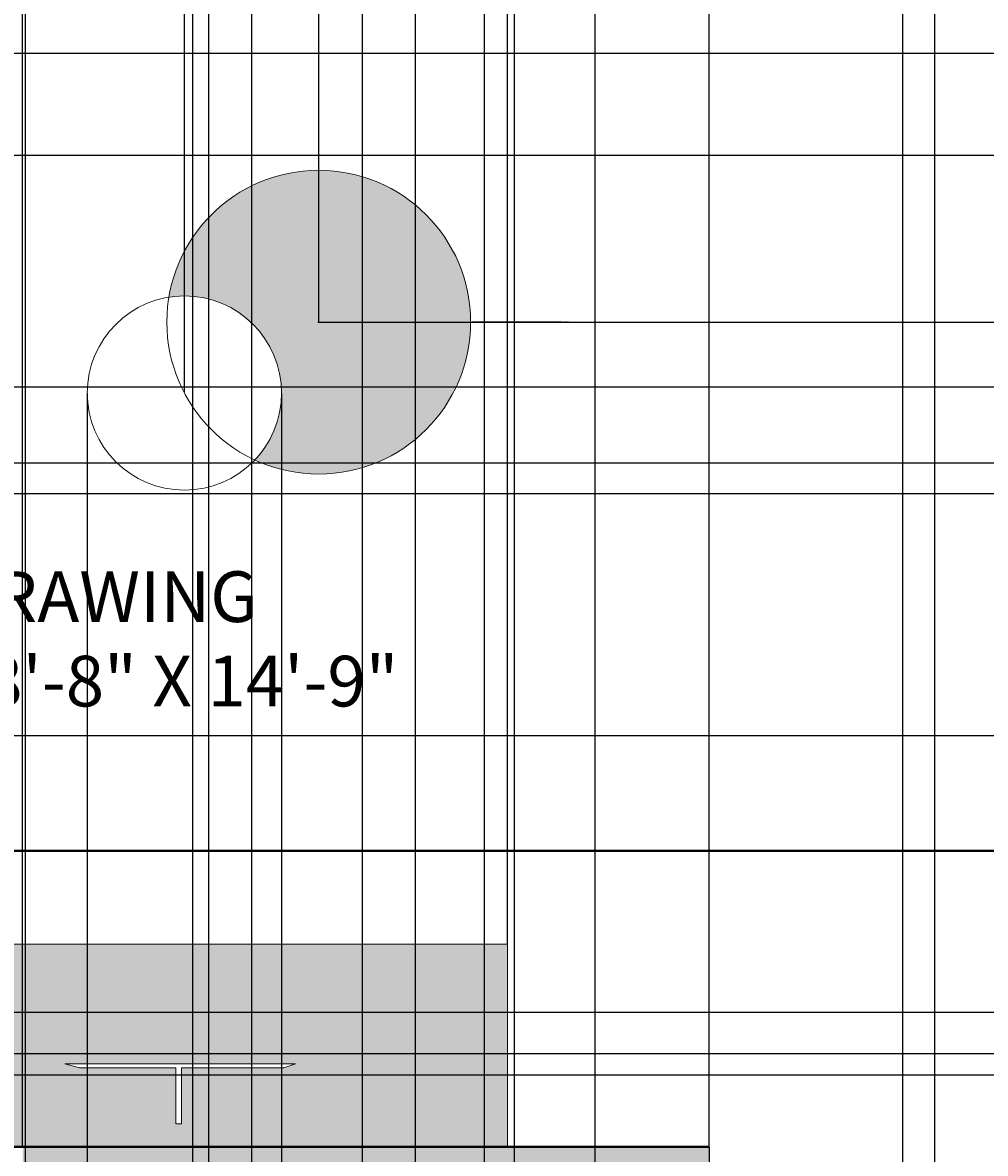
# Model space of a CAD drawing. Units: inches. Extents: x 818 to 1898, y 976 to 2364.
# Tile 24 of 96: x 1284 to 1398, y 1509 to 1643. Entities that reach past the tile are written whole.
import ezdxf

# ---------------------------------------------------------------- set-up
doc = ezdxf.new("R2010")
doc.units = ezdxf.units.IN
doc.header["$LTSCALE"] = 5
doc.header["$MEASUREMENT"] = 0
for name, color, linetype, lineweight in [('A-ANNO-DIMS', 2, 'Continuous', 18), ('A-AREA-IDEN', 7, 'Continuous', 18), ('A-DOOR', 3, 'Continuous', 25), ('A-EQPM', 8, 'Continuous', 18), ('A-FLOR-CASE', 8, 'Continuous', 18), ('A-FLOR-CASE-PATT', 33, 'Continuous', 9), ('A-FURN', 8, 'Continuous', 18), ('A-WALL', 7, 'Continuous', 40)]:
    doc.layers.add(name, color=color, linetype=linetype, lineweight=lineweight)
doc.layers.add('A-WALL-PATT', color=251, linetype='Continuous', lineweight=13, true_color=0x636466)
doc.styles.get("Standard").update_dxf_attribs({"font": 'arial.ttf'})
doc.dimstyles.get("Standard").update_dxf_attribs({"dimtxt": 0.18, "dimasz": 0.18, "dimexe": 0.18, "dimexo": 0.0625, "dimgap": 0.09, "dimtad": 0, "dimtih": 1, "dimtoh": 1, "dimdec": 4, "dimzin": 0, "dimdsep": 46, "dimtxsty": 'Standard', "dimcen": 0.09, "dimadec": 0, "dimazin": 0, "dimtfac": 1, "dimtdec": 4, "dimtofl": 0, "dimtmove": 0, "dimatfit": 3, "dimfxl": 1, "dimtolj": 1, "dimtzin": 0, "dimarcsym": 0})

# ---------------------------------------------------------------- blocks, each defined once
blk = doc.blocks.new('*D61')
at = {"layer": 'A-ANNO-DIMS', "color": 0, "lineweight": -2, "ltscale": 5, "transparency": 16777216}
for p, q in [((1071.73, 1203.03), (1071.73, 2363.87)), ((1071.91, 2363.69), (1250.94, 2363.69)), ((1430.55, 2363.69), (1251.51, 2363.69)), ((1430.73, 1203.03), (1430.73, 2363.87))]:
    blk.add_line(p, q, dxfattribs=at)
at = {"layer": 'A-ANNO-DIMS', "color": 0, "ltscale": 5, "transparency": 16777216}
for points in [[(1071.91, 2363.72), (1071.91, 2363.66), (1071.73, 2363.69)], [(1430.55, 2363.72), (1430.55, 2363.66), (1430.73, 2363.69)]]:
    blk.add_solid(points, dxfattribs=at)
at = {"layer": 'Defpoints', "color": 0, "ltscale": 5, "transparency": 16777216}
for p in [(1430.73, 2363.69), (1071.73, 1202.96), (1430.73, 1202.96)]:
    blk.add_point(p, dxfattribs=at)
at = {"layer": 'A-ANNO-DIMS', "color": 0, "ltscale": 5, "transparency": 16777216, "insert": (1251.23, 2363.69), "char_height": 0.18, "attachment_point": 5}
blk.add_mtext('\\A1;359', dxfattribs=at)
blk = doc.blocks.new('*D64')
at = {"layer": 'A-ANNO-DIMS', "color": 0, "lineweight": -2, "ltscale": 5, "transparency": 16777216}
for p, q in [((1197.73, 1501.14), (1197.73, 2363.87)), ((1197.91, 2363.69), (1313.93, 2363.69)), ((1430.55, 2363.69), (1314.52, 2363.69)), ((1430.73, 1501.14), (1430.73, 2363.87))]:
    blk.add_line(p, q, dxfattribs=at)
at = {"layer": 'A-ANNO-DIMS', "color": 0, "ltscale": 5, "transparency": 16777216}
for points in [[(1197.91, 2363.72), (1197.91, 2363.66), (1197.73, 2363.69)], [(1430.55, 2363.72), (1430.55, 2363.66), (1430.73, 2363.69)]]:
    blk.add_solid(points, dxfattribs=at)
at = {"layer": 'Defpoints', "color": 0, "ltscale": 5, "transparency": 16777216}
for p in [(1430.73, 2363.69), (1197.73, 1501.08), (1430.73, 1501.08)]:
    blk.add_point(p, dxfattribs=at)
at = {"layer": 'A-ANNO-DIMS', "color": 0, "ltscale": 5, "transparency": 16777216, "insert": (1314.23, 2363.69), "char_height": 0.18, "attachment_point": 5}
blk.add_mtext('\\A1;233', dxfattribs=at)
blk = doc.blocks.new('*D96')
at = {"layer": 'A-ANNO-DIMS', "color": 0, "lineweight": -2, "ltscale": 5, "transparency": 16777216}
for p, q in [((1229.65, 1071.12), (1229.65, 2363.87)), ((1229.83, 2363.69), (1256.52, 2363.69)), ((1283.99, 2363.69), (1257.3, 2363.69)), ((1284.17, 1071.12), (1284.17, 2363.87))]:
    blk.add_line(p, q, dxfattribs=at)
at = {"layer": 'A-ANNO-DIMS', "color": 0, "ltscale": 5, "transparency": 16777216}
for points in [[(1229.83, 2363.72), (1229.83, 2363.66), (1229.65, 2363.69)], [(1283.99, 2363.72), (1283.99, 2363.66), (1284.17, 2363.69)]]:
    blk.add_solid(points, dxfattribs=at)
at = {"layer": 'Defpoints', "color": 0, "ltscale": 5, "transparency": 16777216}
for p in [(1284.17, 2363.69), (1229.65, 1071.06), (1284.17, 1071.06)]:
    blk.add_point(p, dxfattribs=at)
at = {"layer": 'A-ANNO-DIMS', "color": 0, "ltscale": 5, "transparency": 16777216, "insert": (1256.91, 2363.69), "char_height": 0.18, "attachment_point": 5}
blk.add_mtext('\\A1;54.52', dxfattribs=at)
blk = doc.blocks.new('*D97')
at = {"layer": 'A-ANNO-DIMS', "color": 0, "lineweight": -2, "ltscale": 5, "transparency": 16777216}
for p, q in [((1284.17, 1071.12), (1284.17, 2363.87)), ((1284.35, 2363.69), (1310.96, 2363.69)), ((1338.36, 2363.69), (1311.75, 2363.69)), ((1338.54, 1071.12), (1338.54, 2363.87))]:
    blk.add_line(p, q, dxfattribs=at)
at = {"layer": 'A-ANNO-DIMS', "color": 0, "ltscale": 5, "transparency": 16777216}
for points in [[(1284.35, 2363.72), (1284.35, 2363.66), (1284.17, 2363.69)], [(1338.36, 2363.72), (1338.36, 2363.66), (1338.54, 2363.69)]]:
    blk.add_solid(points, dxfattribs=at)
at = {"layer": 'Defpoints', "color": 0, "ltscale": 5, "transparency": 16777216}
for p in [(1338.54, 2363.69), (1284.17, 1071.06), (1338.54, 1071.06)]:
    blk.add_point(p, dxfattribs=at)
at = {"layer": 'A-ANNO-DIMS', "color": 0, "ltscale": 5, "transparency": 16777216, "insert": (1311.36, 2363.69), "char_height": 0.18, "attachment_point": 5}
blk.add_mtext('\\A1;54.37', dxfattribs=at)
blk = doc.blocks.new('*D98')
at = {"layer": 'A-ANNO-DIMS', "color": 0, "lineweight": -2, "ltscale": 5, "transparency": 16777216}
for p, q in [((1338.54, 1071.12), (1338.54, 2363.87)), ((1338.72, 2363.69), (1364.81, 2363.69)), ((1391.7, 2363.69), (1365.6, 2363.69)), ((1391.88, 1071.12), (1391.88, 2363.87))]:
    blk.add_line(p, q, dxfattribs=at)
at = {"layer": 'A-ANNO-DIMS', "color": 0, "ltscale": 5, "transparency": 16777216}
for points in [[(1338.72, 2363.72), (1338.72, 2363.66), (1338.54, 2363.69)], [(1391.7, 2363.72), (1391.7, 2363.66), (1391.88, 2363.69)]]:
    blk.add_solid(points, dxfattribs=at)
at = {"layer": 'Defpoints', "color": 0, "ltscale": 5, "transparency": 16777216}
for p in [(1391.88, 2363.69), (1338.54, 1071.06), (1391.88, 1071.06)]:
    blk.add_point(p, dxfattribs=at)
at = {"layer": 'A-ANNO-DIMS', "color": 0, "ltscale": 5, "transparency": 16777216, "insert": (1365.21, 2363.69), "char_height": 0.18, "attachment_point": 5}
blk.add_mtext('\\A1;53.33', dxfattribs=at)
blk = doc.blocks.new('*D99')
at = {"layer": 'A-ANNO-DIMS', "color": 0, "lineweight": -2, "ltscale": 5, "transparency": 16777216}
for p, q in [((1391.88, 1071.12), (1391.88, 2363.87)), ((1392.06, 2363.69), (1420.45, 2363.69)), ((1449.64, 2363.69), (1421.24, 2363.69)), ((1449.82, 1071.12), (1449.82, 2363.87))]:
    blk.add_line(p, q, dxfattribs=at)
at = {"layer": 'A-ANNO-DIMS', "color": 0, "ltscale": 5, "transparency": 16777216}
for points in [[(1392.06, 2363.72), (1392.06, 2363.66), (1391.88, 2363.69)], [(1449.64, 2363.72), (1449.64, 2363.66), (1449.82, 2363.69)]]:
    blk.add_solid(points, dxfattribs=at)
at = {"layer": 'Defpoints', "color": 0, "ltscale": 5, "transparency": 16777216}
for p in [(1449.82, 2363.69), (1391.88, 1071.06), (1449.82, 1071.06)]:
    blk.add_point(p, dxfattribs=at)
at = {"layer": 'A-ANNO-DIMS', "color": 0, "ltscale": 5, "transparency": 16777216, "insert": (1420.85, 2363.69), "char_height": 0.18, "attachment_point": 5}
blk.add_mtext('\\A1;57.94', dxfattribs=at)
blk = doc.blocks.new('*D117')
at = {"layer": 'A-ANNO-DIMS', "color": 0, "lineweight": -2, "ltscale": 5, "transparency": 16777216}
for p, q in [((1766.29, 1545.18), (818.03, 1545.18)), ((818.21, 1545), (818.21, 1501.18)), ((818.21, 1456.99), (818.21, 1500.81)), ((1766.29, 1456.81), (818.03, 1456.81))]:
    blk.add_line(p, q, dxfattribs=at)
at = {"layer": 'A-ANNO-DIMS', "color": 0, "ltscale": 5, "transparency": 16777216}
for points in [[(818.18, 1545), (818.24, 1545), (818.21, 1545.18)], [(818.18, 1456.99), (818.24, 1456.99), (818.21, 1456.81)]]:
    blk.add_solid(points, dxfattribs=at)
at = {"layer": 'Defpoints', "color": 0, "ltscale": 5, "transparency": 16777216}
for p in [(818.21, 1545.18), (1766.35, 1545.18), (1766.35, 1456.81)]:
    blk.add_point(p, dxfattribs=at)
at = {"layer": 'A-ANNO-DIMS', "color": 0, "ltscale": 5, "transparency": 16777216, "insert": (818.21, 1501), "char_height": 0.18, "attachment_point": 5}
blk.add_mtext('\\A1;88.37', dxfattribs=at)
blk = doc.blocks.new('*D118')
at = {"layer": 'A-ANNO-DIMS', "color": 0, "lineweight": -2, "ltscale": 5, "transparency": 16777216}
for p, q in [((1766.29, 1627.51), (818.03, 1627.51)), ((818.21, 1627.33), (818.21, 1586.53)), ((818.21, 1545.36), (818.21, 1586.16)), ((1766.29, 1545.18), (818.03, 1545.18))]:
    blk.add_line(p, q, dxfattribs=at)
at = {"layer": 'A-ANNO-DIMS', "color": 0, "ltscale": 5, "transparency": 16777216}
for points in [[(818.18, 1627.33), (818.24, 1627.33), (818.21, 1627.51)], [(818.18, 1545.36), (818.24, 1545.36), (818.21, 1545.18)]]:
    blk.add_solid(points, dxfattribs=at)
at = {"layer": 'Defpoints', "color": 0, "ltscale": 5, "transparency": 16777216}
for p in [(818.21, 1627.51), (1766.35, 1627.51), (1766.35, 1545.18)]:
    blk.add_point(p, dxfattribs=at)
at = {"layer": 'A-ANNO-DIMS', "color": 0, "ltscale": 5, "transparency": 16777216, "insert": (818.21, 1586.34), "char_height": 0.18, "attachment_point": 5}
blk.add_mtext('\\A1;82.32', dxfattribs=at)
blk = doc.blocks.new('*D119')
at = {"layer": 'A-ANNO-DIMS', "color": 0, "lineweight": -2, "ltscale": 5, "transparency": 16777216}
for p, q in [((1766.29, 1716.99), (818.03, 1716.99)), ((818.21, 1716.81), (818.21, 1672.43)), ((818.21, 1627.69), (818.21, 1672.06)), ((1766.29, 1627.51), (818.03, 1627.51))]:
    blk.add_line(p, q, dxfattribs=at)
at = {"layer": 'A-ANNO-DIMS', "color": 0, "ltscale": 5, "transparency": 16777216}
for points in [[(818.18, 1716.81), (818.24, 1716.81), (818.21, 1716.99)], [(818.18, 1627.69), (818.24, 1627.69), (818.21, 1627.51)]]:
    blk.add_solid(points, dxfattribs=at)
at = {"layer": 'Defpoints', "color": 0, "ltscale": 5, "transparency": 16777216}
for p in [(818.21, 1716.99), (1766.35, 1716.99), (1766.35, 1627.51)]:
    blk.add_point(p, dxfattribs=at)
at = {"layer": 'A-ANNO-DIMS', "color": 0, "ltscale": 5, "transparency": 16777216, "insert": (818.21, 1672.25), "char_height": 0.18, "attachment_point": 5}
blk.add_mtext('\\A1;89.48', dxfattribs=at)
blk = doc.blocks.new('*D159')
at = {"layer": 'A-ANNO-DIMS', "color": 0, "lineweight": -2, "ltscale": 5, "transparency": 16777216}
for p, q in [((1206.73, 1687.02), (1206.73, 975.66)), ((1463.73, 1687.02), (1463.73, 975.66)), ((1206.91, 975.84), (1334.93, 975.84)), ((1463.55, 975.84), (1335.52, 975.84))]:
    blk.add_line(p, q, dxfattribs=at)
at = {"layer": 'A-ANNO-DIMS', "color": 0, "ltscale": 5, "transparency": 16777216}
for points in [[(1206.91, 975.87), (1206.91, 975.81), (1206.73, 975.84)], [(1463.55, 975.87), (1463.55, 975.81), (1463.73, 975.84)]]:
    blk.add_solid(points, dxfattribs=at)
at = {"layer": 'Defpoints', "color": 0, "ltscale": 5, "transparency": 16777216}
for p in [(1206.73, 1687.08), (1463.73, 1687.08), (1463.73, 975.84)]:
    blk.add_point(p, dxfattribs=at)
at = {"layer": 'A-ANNO-DIMS', "color": 0, "ltscale": 5, "transparency": 16777216, "insert": (1335.23, 975.84), "char_height": 0.18, "attachment_point": 5}
blk.add_mtext('\\A1;257', dxfattribs=at)
blk = doc.blocks.new('*D165')
at = {"layer": 'A-ANNO-DIMS', "color": 0, "lineweight": -2, "ltscale": 5, "transparency": 16777216}
for p, q in [((1283.82, 1510.14), (1283.82, 2363.87)), ((1284, 2363.69), (1324.09, 2363.69)), ((1364.97, 2363.69), (1324.88, 2363.69)), ((1365.15, 1510.14), (1365.15, 2363.87))]:
    blk.add_line(p, q, dxfattribs=at)
at = {"layer": 'A-ANNO-DIMS', "color": 0, "ltscale": 5, "transparency": 16777216}
for points in [[(1284, 2363.72), (1284, 2363.66), (1283.82, 2363.69)], [(1364.97, 2363.72), (1364.97, 2363.66), (1365.15, 2363.69)]]:
    blk.add_solid(points, dxfattribs=at)
at = {"layer": 'Defpoints', "color": 0, "ltscale": 5, "transparency": 16777216}
for p in [(1365.15, 2363.69), (1283.82, 1510.08), (1365.15, 1510.08)]:
    blk.add_point(p, dxfattribs=at)
at = {"layer": 'A-ANNO-DIMS', "color": 0, "ltscale": 5, "transparency": 16777216, "insert": (1324.48, 2363.69), "char_height": 0.18, "attachment_point": 5}
blk.add_mtext('\\A1;81.33', dxfattribs=at)
blk = doc.blocks.new('*D181')
at = {"layer": 'A-ANNO-DIMS', "color": 0, "lineweight": -2, "ltscale": 5, "transparency": 16777216}
for p, q in [((1599.66, 1639.58), (818.03, 1639.58)), ((818.21, 1639.4), (818.21, 1620.01)), ((818.21, 1600.26), (818.21, 1619.65)), ((1619.66, 1600.08), (818.03, 1600.08))]:
    blk.add_line(p, q, dxfattribs=at)
at = {"layer": 'A-ANNO-DIMS', "color": 0, "ltscale": 5, "transparency": 16777216}
for points in [[(818.18, 1639.4), (818.24, 1639.4), (818.21, 1639.58)], [(818.18, 1600.26), (818.24, 1600.26), (818.21, 1600.08)]]:
    blk.add_solid(points, dxfattribs=at)
at = {"layer": 'Defpoints', "color": 0, "ltscale": 5, "transparency": 16777216}
for p in [(1599.73, 1639.58), (818.21, 1600.08), (1619.73, 1600.08)]:
    blk.add_point(p, dxfattribs=at)
at = {"layer": 'A-ANNO-DIMS', "color": 0, "ltscale": 5, "transparency": 16777216, "insert": (818.21, 1619.83), "char_height": 0.18, "attachment_point": 5}
blk.add_mtext('\\A1;39.5', dxfattribs=at)
blk = doc.blocks.new('*D187')
at = {"layer": 'A-ANNO-DIMS', "color": 0, "lineweight": -2, "ltscale": 5, "transparency": 16777216}
for p, q in [((1705.66, 1545.08), (818.03, 1545.08)), ((818.21, 1544.9), (818.21, 1533.26)), ((818.21, 1521.26), (818.21, 1532.9)), ((1705.66, 1521.08), (818.03, 1521.08))]:
    blk.add_line(p, q, dxfattribs=at)
at = {"layer": 'A-ANNO-DIMS', "color": 0, "ltscale": 5, "transparency": 16777216}
for points in [[(818.18, 1544.9), (818.24, 1544.9), (818.21, 1545.08)], [(818.18, 1521.26), (818.24, 1521.26), (818.21, 1521.08)]]:
    blk.add_solid(points, dxfattribs=at)
at = {"layer": 'Defpoints', "color": 0, "ltscale": 5, "transparency": 16777216}
for p in [(818.21, 1545.08), (1705.73, 1545.08), (1705.73, 1521.08)]:
    blk.add_point(p, dxfattribs=at)
at = {"layer": 'A-ANNO-DIMS', "color": 0, "ltscale": 5, "transparency": 16777216, "insert": (818.21, 1533.08), "char_height": 0.18, "attachment_point": 5}
blk.add_mtext('\\A1;24', dxfattribs=at)
blk = doc.blocks.new('*D194')
at = {"layer": 'A-ANNO-DIMS', "color": 0, "lineweight": -2, "ltscale": 5, "transparency": 16777216}
for p, q in [((1616.66, 1591.08), (818.03, 1591.08)), ((818.21, 1590.9), (818.21, 1575.1)), ((818.21, 1558.93), (818.21, 1574.73)), ((1616.66, 1558.75), (818.03, 1558.75))]:
    blk.add_line(p, q, dxfattribs=at)
at = {"layer": 'A-ANNO-DIMS', "color": 0, "ltscale": 5, "transparency": 16777216}
for points in [[(818.18, 1590.9), (818.24, 1590.9), (818.21, 1591.08)], [(818.18, 1558.93), (818.24, 1558.93), (818.21, 1558.75)]]:
    blk.add_solid(points, dxfattribs=at)
at = {"layer": 'Defpoints', "color": 0, "ltscale": 5, "transparency": 16777216}
for p in [(818.21, 1591.08), (1616.73, 1591.08), (1616.73, 1558.75)]:
    blk.add_point(p, dxfattribs=at)
at = {"layer": 'A-ANNO-DIMS', "color": 0, "ltscale": 5, "transparency": 16777216, "insert": (818.21, 1574.92), "char_height": 0.18, "attachment_point": 5}
blk.add_mtext('\\A1;32.326', dxfattribs=at)
blk = doc.blocks.new('*D201')
at = {"layer": 'A-ANNO-DIMS', "color": 0, "lineweight": -2, "ltscale": 5, "transparency": 16777216}
for p, q in [((1678.27, 1518.56), (818.03, 1518.56)), ((818.21, 1518.38), (818.21, 1498.18)), ((818.21, 1477.61), (818.21, 1497.81)), ((1678.27, 1477.43), (818.03, 1477.43))]:
    blk.add_line(p, q, dxfattribs=at)
at = {"layer": 'A-ANNO-DIMS', "color": 0, "ltscale": 5, "transparency": 16777216}
for points in [[(818.18, 1518.38), (818.24, 1518.38), (818.21, 1518.56)], [(818.18, 1477.61), (818.24, 1477.61), (818.21, 1477.43)]]:
    blk.add_solid(points, dxfattribs=at)
at = {"layer": 'Defpoints', "color": 0, "ltscale": 5, "transparency": 16777216}
for p in [(818.21, 1518.56), (1678.33, 1518.56), (1678.33, 1477.43)]:
    blk.add_point(p, dxfattribs=at)
at = {"layer": 'A-ANNO-DIMS', "color": 0, "ltscale": 5, "transparency": 16777216, "insert": (818.21, 1497.99), "char_height": 0.18, "attachment_point": 5}
blk.add_mtext('\\A1;41.135', dxfattribs=at)
blk = doc.blocks.new('*D231')
at = {"layer": 'A-ANNO-DIMS', "color": 0, "lineweight": -2, "ltscale": 5, "transparency": 16777216}
for p, q in [((1303.93, 1952.98), (1303.93, 975.66)), ((1402.52, 1952.98), (1402.52, 975.66)), ((1304.11, 975.84), (1352.83, 975.84)), ((1402.34, 975.84), (1353.62, 975.84))]:
    blk.add_line(p, q, dxfattribs=at)
at = {"layer": 'A-ANNO-DIMS', "color": 0, "ltscale": 5, "transparency": 16777216}
for points in [[(1304.11, 975.87), (1304.11, 975.81), (1303.93, 975.84)], [(1402.34, 975.87), (1402.34, 975.81), (1402.52, 975.84)]]:
    blk.add_solid(points, dxfattribs=at)
at = {"layer": 'Defpoints', "color": 0, "ltscale": 5, "transparency": 16777216}
for p in [(1303.93, 1953.04), (1402.52, 1953.04), (1402.52, 975.84)]:
    blk.add_point(p, dxfattribs=at)
at = {"layer": 'A-ANNO-DIMS', "color": 0, "ltscale": 5, "transparency": 16777216, "insert": (1353.22, 975.84), "char_height": 0.18, "attachment_point": 5}
blk.add_mtext('\\A1;98.59', dxfattribs=at)
blk = doc.blocks.new('*D233')
at = {"layer": 'A-ANNO-DIMS', "color": 0, "lineweight": -2, "ltscale": 5, "transparency": 16777216}
for p, q in [((1267.73, 2044.02), (1267.73, 975.66)), ((1303.93, 2008.33), (1303.93, 975.66)), ((1267.91, 975.84), (1285.36, 975.84)), ((1303.75, 975.84), (1286.29, 975.84))]:
    blk.add_line(p, q, dxfattribs=at)
at = {"layer": 'A-ANNO-DIMS', "color": 0, "ltscale": 5, "transparency": 16777216}
for points in [[(1267.91, 975.87), (1267.91, 975.81), (1267.73, 975.84)], [(1303.75, 975.87), (1303.75, 975.81), (1303.93, 975.84)]]:
    blk.add_solid(points, dxfattribs=at)
at = {"layer": 'Defpoints', "color": 0, "ltscale": 5, "transparency": 16777216}
for p in [(1267.73, 2044.08), (1303.93, 2008.39), (1303.93, 975.84)]:
    blk.add_point(p, dxfattribs=at)
at = {"layer": 'A-ANNO-DIMS', "color": 0, "ltscale": 5, "transparency": 16777216, "insert": (1285.83, 975.84), "char_height": 0.18, "attachment_point": 5}
blk.add_mtext('\\A1;36.206', dxfattribs=at)
blk = doc.blocks.new('*D236')
at = {"layer": 'A-ANNO-DIMS', "color": 0, "lineweight": -2, "ltscale": 5, "transparency": 16777216}
for p, q in [((1310.91, 2026.14), (1310.91, 975.66)), ((1342.04, 2026.14), (1342.04, 975.66)), ((1311.09, 975.84), (1326.08, 975.84)), ((1341.86, 975.84), (1326.87, 975.84))]:
    blk.add_line(p, q, dxfattribs=at)
at = {"layer": 'A-ANNO-DIMS', "color": 0, "ltscale": 5, "transparency": 16777216}
for points in [[(1311.09, 975.87), (1311.09, 975.81), (1310.91, 975.84)], [(1341.86, 975.87), (1341.86, 975.81), (1342.04, 975.84)]]:
    blk.add_solid(points, dxfattribs=at)
at = {"layer": 'Defpoints', "color": 0, "ltscale": 5, "transparency": 16777216}
for p in [(1310.91, 2026.21), (1342.04, 2026.21), (1342.04, 975.84)]:
    blk.add_point(p, dxfattribs=at)
at = {"layer": 'A-ANNO-DIMS', "color": 0, "ltscale": 5, "transparency": 16777216, "insert": (1326.48, 975.84), "char_height": 0.18, "attachment_point": 5}
blk.add_mtext('\\A1;31.14', dxfattribs=at)
blk = doc.blocks.new('*D245')
at = {"layer": 'A-ANNO-DIMS', "color": 0, "lineweight": -2, "ltscale": 5, "transparency": 16777216}
for p, q in [((1291.48, 1599.31), (1291.48, 975.66)), ((1314.49, 1599.31), (1314.49, 975.66)), ((1291.66, 975.84), (1302.61, 975.84)), ((1314.31, 975.84), (1303.36, 975.84))]:
    blk.add_line(p, q, dxfattribs=at)
at = {"layer": 'A-ANNO-DIMS', "color": 0, "ltscale": 5, "transparency": 16777216}
for points in [[(1291.66, 975.87), (1291.66, 975.81), (1291.48, 975.84)], [(1314.31, 975.87), (1314.31, 975.81), (1314.49, 975.84)]]:
    blk.add_solid(points, dxfattribs=at)
at = {"layer": 'Defpoints', "color": 0, "ltscale": 5, "transparency": 16777216}
for p in [(1291.48, 1599.37), (1314.49, 1599.37), (1314.49, 975.84)]:
    blk.add_point(p, dxfattribs=at)
at = {"layer": 'A-ANNO-DIMS', "color": 0, "ltscale": 5, "transparency": 16777216, "insert": (1302.98, 975.84), "char_height": 0.18, "attachment_point": 5}
blk.add_mtext('\\A1;23.01', dxfattribs=at)
blk = doc.blocks.new('*D252')
at = {"layer": 'A-ANNO-DIMS', "color": 0, "lineweight": -2, "ltscale": 5, "transparency": 16777216}
for p, q in [((1330.3, 2053.02), (1330.3, 975.66)), ((1388.03, 2053.02), (1388.03, 975.66)), ((1330.48, 975.84), (1358.77, 975.84)), ((1387.85, 975.84), (1359.56, 975.84))]:
    blk.add_line(p, q, dxfattribs=at)
at = {"layer": 'A-ANNO-DIMS', "color": 0, "ltscale": 5, "transparency": 16777216}
for points in [[(1330.48, 975.87), (1330.48, 975.81), (1330.3, 975.84)], [(1387.85, 975.87), (1387.85, 975.81), (1388.03, 975.84)]]:
    blk.add_solid(points, dxfattribs=at)
at = {"layer": 'Defpoints', "color": 0, "ltscale": 5, "transparency": 16777216}
for p in [(1330.3, 2053.08), (1388.03, 2053.08), (1388.03, 975.84)]:
    blk.add_point(p, dxfattribs=at)
at = {"layer": 'A-ANNO-DIMS', "color": 0, "ltscale": 5, "transparency": 16777216, "insert": (1359.17, 975.84), "char_height": 0.18, "attachment_point": 5}
blk.add_mtext('\\A1;57.73', dxfattribs=at)
blk = doc.blocks.new('*D254')
at = {"layer": 'A-ANNO-DIMS', "color": 0, "lineweight": -2, "ltscale": 5, "transparency": 16777216}
for p, q in [((1267.73, 2044.02), (1267.73, 975.66)), ((1330.3, 2044.02), (1330.3, 975.66)), ((1267.91, 975.84), (1298.62, 975.84)), ((1330.12, 975.84), (1299.41, 975.84))]:
    blk.add_line(p, q, dxfattribs=at)
at = {"layer": 'A-ANNO-DIMS', "color": 0, "ltscale": 5, "transparency": 16777216}
for points in [[(1267.91, 975.87), (1267.91, 975.81), (1267.73, 975.84)], [(1330.12, 975.87), (1330.12, 975.81), (1330.3, 975.84)]]:
    blk.add_solid(points, dxfattribs=at)
at = {"layer": 'Defpoints', "color": 0, "ltscale": 5, "transparency": 16777216}
for p in [(1267.73, 2044.08), (1330.3, 2044.08), (1330.3, 975.84)]:
    blk.add_point(p, dxfattribs=at)
at = {"layer": 'A-ANNO-DIMS', "color": 0, "ltscale": 5, "transparency": 16777216, "insert": (1299.02, 975.84), "char_height": 0.18, "attachment_point": 5}
blk.add_mtext('\\A1;62.58', dxfattribs=at)
blk = doc.blocks.new('*D269')
at = {"layer": 'A-ANNO-DIMS', "color": 0, "lineweight": -2, "ltscale": 5, "transparency": 16777216}
for p, q in [((1246.94, 1534.14), (1246.94, 2363.87)), ((1247.12, 2363.69), (1293.71, 2363.69)), ((1341.08, 2363.69), (1294.49, 2363.69)), ((1341.26, 1534.14), (1341.26, 2363.87))]:
    blk.add_line(p, q, dxfattribs=at)
at = {"layer": 'A-ANNO-DIMS', "color": 0, "ltscale": 5, "transparency": 16777216}
for points in [[(1247.12, 2363.72), (1247.12, 2363.66), (1246.94, 2363.69)], [(1341.08, 2363.72), (1341.08, 2363.66), (1341.26, 2363.69)]]:
    blk.add_solid(points, dxfattribs=at)
at = {"layer": 'Defpoints', "color": 0, "ltscale": 5, "transparency": 16777216}
for p in [(1341.26, 2363.69), (1246.94, 1534.08), (1341.26, 1534.08)]:
    blk.add_point(p, dxfattribs=at)
at = {"layer": 'A-ANNO-DIMS', "color": 0, "ltscale": 5, "transparency": 16777216, "insert": (1294.1, 2363.69), "char_height": 0.18, "attachment_point": 5}
blk.add_mtext('\\A1;94.32', dxfattribs=at)
blk = doc.blocks.new('*D272')
at = {"layer": 'A-ANNO-DIMS', "color": 0, "lineweight": -2, "ltscale": 5, "transparency": 16777216}
for p, q in [((1406.66, 1587.42), (818.03, 1587.42)), ((818.21, 1587.24), (818.21, 1556.89)), ((818.21, 1526.18), (818.21, 1556.52)), ((1406.66, 1526), (818.03, 1526))]:
    blk.add_line(p, q, dxfattribs=at)
at = {"layer": 'A-ANNO-DIMS', "color": 0, "ltscale": 5, "transparency": 16777216}
for points in [[(818.18, 1587.24), (818.24, 1587.24), (818.21, 1587.42)], [(818.18, 1526.18), (818.24, 1526.18), (818.21, 1526)]]:
    blk.add_solid(points, dxfattribs=at)
at = {"layer": 'Defpoints', "color": 0, "ltscale": 5, "transparency": 16777216}
for p in [(818.21, 1587.42), (1406.73, 1587.42), (1406.73, 1526)]:
    blk.add_point(p, dxfattribs=at)
at = {"layer": 'A-ANNO-DIMS', "color": 0, "ltscale": 5, "transparency": 16777216, "insert": (818.21, 1556.71), "char_height": 0.18, "attachment_point": 5}
blk.add_mtext('\\A1;61.42', dxfattribs=at)
blk = doc.blocks.new('*D278')
at = {"layer": 'A-ANNO-DIMS', "color": 0, "lineweight": -2, "ltscale": 5, "transparency": 16777216}
for p, q in [((1324.03, 1700.74), (1324.03, 975.66)), ((1267.73, 1696.02), (1267.73, 975.66)), ((1267.91, 975.84), (1295.5, 975.84)), ((1323.85, 975.84), (1296.26, 975.84))]:
    blk.add_line(p, q, dxfattribs=at)
at = {"layer": 'A-ANNO-DIMS', "color": 0, "ltscale": 5, "transparency": 16777216}
for points in [[(1267.91, 975.87), (1267.91, 975.81), (1267.73, 975.84)], [(1323.85, 975.87), (1323.85, 975.81), (1324.03, 975.84)]]:
    blk.add_solid(points, dxfattribs=at)
at = {"layer": 'Defpoints', "color": 0, "ltscale": 5, "transparency": 16777216}
for p in [(1324.03, 1700.81), (1267.73, 1696.08), (1324.03, 975.84)]:
    blk.add_point(p, dxfattribs=at)
at = {"layer": 'A-ANNO-DIMS', "color": 0, "ltscale": 5, "transparency": 16777216, "insert": (1295.88, 975.84), "char_height": 0.18, "attachment_point": 5}
blk.add_mtext('\\A1;56.31', dxfattribs=at)
blk = doc.blocks.new('*D283')
at = {"layer": 'A-ANNO-DIMS', "color": 0, "lineweight": -2, "ltscale": 5, "transparency": 16777216}
for p, q in [((1351.6, 1761.39), (1351.6, 975.66)), ((1267.73, 1696.02), (1267.73, 975.66)), ((1267.91, 975.84), (1309.27, 975.84)), ((1351.42, 975.84), (1310.06, 975.84))]:
    blk.add_line(p, q, dxfattribs=at)
at = {"layer": 'A-ANNO-DIMS', "color": 0, "ltscale": 5, "transparency": 16777216}
for points in [[(1267.91, 975.87), (1267.91, 975.81), (1267.73, 975.84)], [(1351.42, 975.87), (1351.42, 975.81), (1351.6, 975.84)]]:
    blk.add_solid(points, dxfattribs=at)
at = {"layer": 'Defpoints', "color": 0, "ltscale": 5, "transparency": 16777216}
for p in [(1351.6, 1761.45), (1267.73, 1696.08), (1351.6, 975.84)]:
    blk.add_point(p, dxfattribs=at)
at = {"layer": 'A-ANNO-DIMS', "color": 0, "ltscale": 5, "transparency": 16777216, "insert": (1309.66, 975.84), "char_height": 0.18, "attachment_point": 5}
blk.add_mtext('\\A1;83.87', dxfattribs=at)
blk = doc.blocks.new('*D285')
at = {"layer": 'A-ANNO-DIMS', "color": 0, "lineweight": -2, "ltscale": 5, "transparency": 16777216}
for p, q in [((1305.83, 1830.02), (1305.83, 975.66)), ((1267.73, 1814.9), (1267.73, 975.66)), ((1267.91, 975.84), (1286.47, 975.84)), ((1305.65, 975.84), (1287.08, 975.84))]:
    blk.add_line(p, q, dxfattribs=at)
at = {"layer": 'A-ANNO-DIMS', "color": 0, "ltscale": 5, "transparency": 16777216}
for points in [[(1267.91, 975.87), (1267.91, 975.81), (1267.73, 975.84)], [(1305.65, 975.87), (1305.65, 975.81), (1305.83, 975.84)]]:
    blk.add_solid(points, dxfattribs=at)
at = {"layer": 'Defpoints', "color": 0, "ltscale": 5, "transparency": 16777216}
for p in [(1305.83, 1830.08), (1267.73, 1814.97), (1267.73, 975.84)]:
    blk.add_point(p, dxfattribs=at)
at = {"layer": 'A-ANNO-DIMS', "color": 0, "ltscale": 5, "transparency": 16777216, "insert": (1286.78, 975.84), "char_height": 0.18, "attachment_point": 5}
blk.add_mtext('\\A1;38.1', dxfattribs=at)
blk = doc.blocks.new('*D290')
at = {"layer": 'A-ANNO-DIMS', "color": 0, "lineweight": -2, "ltscale": 5, "transparency": 16777216}
for p, q in [((1302.98, 1599.43), (1302.98, 2363.87)), ((1303.16, 2363.69), (1310.57, 2363.69)), ((1318.71, 2363.69), (1311.31, 2363.69)), ((1318.89, 1607.83), (1318.89, 2363.87))]:
    blk.add_line(p, q, dxfattribs=at)
at = {"layer": 'A-ANNO-DIMS', "color": 0, "ltscale": 5, "transparency": 16777216}
for points in [[(1303.16, 2363.72), (1303.16, 2363.66), (1302.98, 2363.69)], [(1318.71, 2363.72), (1318.71, 2363.66), (1318.89, 2363.69)]]:
    blk.add_solid(points, dxfattribs=at)
at = {"layer": 'Defpoints', "color": 0, "ltscale": 5, "transparency": 16777216}
for p in [(1318.89, 2363.69), (1318.89, 1607.77), (1302.98, 1599.37)]:
    blk.add_point(p, dxfattribs=at)
at = {"layer": 'A-ANNO-DIMS', "color": 0, "ltscale": 5, "transparency": 16777216, "insert": (1310.94, 2363.69), "char_height": 0.18, "attachment_point": 5}
blk.add_mtext('\\A1;15.91', dxfattribs=at)
blk = doc.blocks.new('*D291')
at = {"layer": 'A-ANNO-DIMS', "color": 0, "lineweight": -2, "ltscale": 5, "transparency": 16777216}
for p, q in [((1206.79, 1687.08), (1897.92, 1687.08)), ((1897.74, 1686.9), (1897.74, 1647.61)), ((1897.74, 1607.95), (1897.74, 1647.24)), ((1318.96, 1607.77), (1897.92, 1607.77))]:
    blk.add_line(p, q, dxfattribs=at)
at = {"layer": 'A-ANNO-DIMS', "color": 0, "ltscale": 5, "transparency": 16777216}
for points in [[(1897.71, 1686.9), (1897.77, 1686.9), (1897.74, 1687.08)], [(1897.71, 1607.95), (1897.77, 1607.95), (1897.74, 1607.77)]]:
    blk.add_solid(points, dxfattribs=at)
at = {"layer": 'Defpoints', "color": 0, "ltscale": 5, "transparency": 16777216}
for p in [(1206.73, 1687.08), (1897.74, 1687.08), (1318.89, 1607.77)]:
    blk.add_point(p, dxfattribs=at)
at = {"layer": 'A-ANNO-DIMS', "color": 0, "ltscale": 5, "transparency": 16777216, "insert": (1897.74, 1647.42), "char_height": 0.18, "attachment_point": 5}
blk.add_mtext('\\A1;79.3', dxfattribs=at)
blk = doc.blocks.new('*D293')
at = {"layer": 'A-ANNO-DIMS', "color": 0, "lineweight": -2, "ltscale": 5, "transparency": 16777216}
for p, q in [((1318.8, 1607.77), (1318.98, 1607.77)), ((1318.89, 1607.68), (1318.89, 1607.86)), ((1347.68, 1607.77), (1337.06, 1607.77))]:
    blk.add_line(p, q, dxfattribs=at)
at = {"layer": 'A-ANNO-DIMS', "color": 0, "ltscale": 5, "transparency": 16777216}
blk.add_solid([(1337.06, 1607.8), (1337.06, 1607.74), (1336.88, 1607.77)], dxfattribs=at)
at = {"layer": 'Defpoints', "color": 0, "ltscale": 5, "transparency": 16777216}
for p in [(1300.9, 1607.77), (1336.88, 1607.77)]:
    blk.add_point(p, dxfattribs=at)
at = {"layer": 'A-ANNO-DIMS', "color": 0, "ltscale": 5, "transparency": 16777216, "insert": (1348.17, 1607.77), "char_height": 0.18, "attachment_point": 5}
blk.add_mtext('\\A1;∅35.98', dxfattribs=at)

msp = doc.modelspace()

# ---------------------------------------------------------------- hatches: boundary and pattern name
at = {"layer": 'A-FLOR-CASE-PATT', "ltscale": 5}
h = msp.add_hatch(color=256, dxfattribs=at)
h.dxf.hatch_style = 1
h.paths.add_polyline_path([(1705.7251, 1941.0782), (1681.7252, 1941.0782), (1681.7252, 1900.0782), (1599.7251, 1900.0782), (1599.7251, 1876.0782), (1705.7251, 1876.0782)])
h.paths.add_polyline_path([(1457.7252, 1409.1177), (1457.7252, 1526.6712), (1439.7252, 1526.6712), (1439.7252, 1457.5313), (1446.3307, 1457.5313), (1446.3307, 1468.9514), (1446.8307, 1470.665), (1446.8307, 1469.665), (1446.8307, 1468.9514), (1446.8307, 1456.8361), (1446.8307, 1444.7258), (1446.8307, 1443.3338), (1446.3307, 1444.7258), (1446.3307, 1456.8361), (1439.7252, 1456.8361), (1439.7252, 1355.0782), (1463.7251, 1355.0782), (1463.7251, 1367.3287), (1458.0475, 1367.3287, -0.23606798), (1457.0475, 1369.3287), (1456.0475, 1369.3287, -0.11764706), (1456.0475, 1386.3287), (1457.0475, 1386.3287, -0.23606798), (1458.0475, 1388.3287), (1463.7251, 1388.3287), (1463.7251, 1389.3211)])
h.paths.add_polyline_path([(1341.2593, 1534.0782), (1246.9377, 1534.0782), (1246.9377, 1510.0782), (1341.2593, 1510.0782)])
h.paths.add_polyline_path([(1288.8272, 1519.927), (1289.8272, 1519.927), (1290.5408, 1519.927), (1302.6561, 1519.927), (1314.7664, 1519.927), (1316.1584, 1519.927), (1314.7664, 1519.427), (1302.6561, 1519.427), (1302.6561, 1512.8214), (1301.9609, 1512.8214), (1301.9609, 1519.427), (1290.5408, 1519.427)], flags=16)
h.paths.add_polyline_path([(1377.7791, 1867.0782), (1344.5531, 1867.0782), (1344.5531, 1860.4726), (1355.9731, 1860.4726), (1357.6867, 1859.9726), (1356.6867, 1859.9726), (1355.9731, 1859.9726), (1343.8579, 1859.9726), (1331.7475, 1859.9726), (1330.3556, 1859.9726), (1331.7475, 1860.4726), (1343.8579, 1860.4726), (1343.8579, 1867.0782), (1311.3271, 1867.0782), (1311.3271, 1853.7496), (1377.7791, 1853.7496)])
h.paths.add_polyline_path([(1301.148, 1610.7299, -0.46196039), (1314.4882, 1599.3725, -0.19222541), (1311.3254, 1591.4497, 0.54791519), (1336.8832, 1607.7707, 0.92061359)])
h.paths.add_polyline_path([(1370.719, 1780.5695, 1), (1332.478, 1780.5695, 1)])
h.paths.add_polyline_path([(1705.7251, 1463.0782), (1681.7252, 1463.0782), (1681.7252, 1379.0782), (1622.7252, 1379.0782), (1622.7252, 1355.0782), (1705.7251, 1355.0782)])
h.paths.add_polyline_path([(1658.1052, 1359.2188), (1658.1786, 1359.2188), (1658.1786, 1373.8763), (1658.1052, 1373.9202)], flags=16)
h.paths.add_polyline_path([(1686.9271, 1409.9311), (1686.8832, 1409.8578), (1701.5845, 1409.8578), (1701.5845, 1409.9311)], flags=16)
h.paths.add_polyline_path([(1637.1266, 1359.2188), (1637.2, 1359.2188), (1637.2, 1373.8763), (1637.1266, 1373.9202)], flags=16)
at = {"layer": 'A-WALL-PATT', "ltscale": 5}
h = msp.add_hatch(color=256, dxfattribs=at)
h.dxf.hatch_style = 1
h.paths.add_polyline_path([(1206.7251, 1687.0782), (1206.7251, 1700.0782), (1197.7251, 1700.0782), (1197.7251, 1501.0782), (1206.7251, 1501.0782), (1206.7251, 1510.0782)])
h.paths.add_polyline_path([(1197.7251, 1590.7585), (1173.7252, 1590.7585), (1173.7252, 1586.7585), (1197.7251, 1586.7585)])
h.paths.add_polyline_path([(1197.7251, 1534.6024), (1173.7252, 1534.6024), (1173.7252, 1530.6024), (1197.7251, 1530.6024)])
h.paths.add_polyline_path([(1365.1463, 1510.0782), (1283.8183, 1510.0782), (1283.8183, 1501.0782), (1365.1463, 1501.0782)])
h.paths.add_polyline_path([(1439.7252, 1591.0782), (1441.7252, 1591.0782), (1441.7252, 1600.0782), (1430.7251, 1600.0782), (1430.7251, 1510.0782), (1406.7251, 1510.0782), (1401.1463, 1510.0782), (1401.1463, 1501.0782), (1430.7251, 1501.0782), (1430.7251, 1486.2383), (1430.7251, 1409.0522), (1439.7252, 1409.0522)])

# ---------------------------------------------------------------- linework, layer by layer
at = {"layer": 'A-DOOR'}
msp.add_line((1365.1463, 1510.0782), (1365.1463, 1501.0782), dxfattribs=at)
at = {"layer": 'A-EQPM'}
for p, q in [((1289.8272, 1519.927), (1288.8272, 1519.927)), ((1288.8272, 1519.927), (1290.5408, 1519.427)), ((1290.5408, 1519.927), (1289.8272, 1519.927)), ((1302.6561, 1519.927), (1290.5408, 1519.927)), ((1301.9609, 1519.427), (1290.5408, 1519.427)), ((1302.6561, 1519.927), (1314.7664, 1519.927)), ((1302.6561, 1519.427), (1314.7664, 1519.427)), ((1314.7664, 1519.927), (1316.1584, 1519.927)), ((1316.1584, 1519.927), (1314.7664, 1519.427))]:
    msp.add_line(p, q, dxfattribs=at)
msp.add_lwpolyline([(1302.6561, 1519.427), (1302.6561, 1512.8214), (1301.9609, 1512.8214), (1301.9609, 1519.427)], dxfattribs=at)
at = {"layer": 'A-FLOR-CASE'}
for p in [(1246.9377, 1534.0782), (1341.2593, 1510.0782)]:
    msp.add_line(p, (1341.2593, 1534.0782), dxfattribs=at)
at = {"layer": 'A-FURN'}
for centre, radius in [((1318.8931, 1607.7707), 17.9901), ((1302.9835, 1599.3725), 11.5048)]:
    msp.add_circle(centre, radius, dxfattribs=at)
at = {"layer": 'A-WALL'}
msp.add_line((1206.7251, 1510.0782), (1365.1463, 1510.0782), dxfattribs=at)

# ---------------------------------------------------------------- texts
at = {"layer": 'A-AREA-IDEN', "ltscale": 5, "insert": (1274.7264, 1578.2498), "char_height": 6, "attachment_point": 1}
msp.add_mtext_dynamic_manual_height_columns('DRAWING\\P18\'-8" X 14\'-9"', width=118.992422, gutter_width=1, heights=[0], dxfattribs=at)

# ---------------------------------------------------------------- dimensions: what is measured, and where the dimension line sits
at = {"layer": 'A-ANNO-DIMS', "ltscale": 5}
for base, p1, p2, override, picture, middle in [((1430.7251, 2363.6929), (1071.7251, 1202.9642), (1430.7251, 1202.9642), {"dimdec": 0, "dimlfac": 1, "dimrnd": 0, "dimzin": 0, "dimdsep": 46, "dimlunit": 2}, '*D61', (1251.2251, 2363.6929)), ((1430.7251, 2363.6929), (1197.7251, 1501.0782), (1430.7251, 1501.0782), {"dimdec": 0, "dimlfac": 1, "dimrnd": 0, "dimzin": 0, "dimdsep": 46, "dimlunit": 2}, '*D64', (1314.2251, 2363.6929)), ((1284.1697, 2363.6929), (1229.6474, 1071.0552), (1284.1697, 1071.0552), {"dimdec": 2, "dimlfac": 1, "dimrnd": 0, "dimzin": 0, "dimdsep": 46, "dimlunit": 2}, '*D96', (1256.9085, 2363.6929)), ((1341.2593, 2363.6929), (1246.9377, 1534.0782), (1341.2593, 1534.0782), {"dimdec": 2, "dimlfac": 1, "dimrnd": 0, "dimzin": 0, "dimdsep": 46, "dimlunit": 2}, '*D269', (1294.0985, 2363.6929)), ((1365.1463, 2363.6929), (1283.8183, 1510.0782), (1365.1463, 1510.0782), {"dimdec": 2, "dimlfac": 1, "dimrnd": 0, "dimzin": 0, "dimdsep": 46, "dimlunit": 2}, '*D165', (1324.4823, 2363.6929)), ((1338.5412, 2363.6929), (1284.1697, 1071.0552), (1338.5412, 1071.0552), {"dimdec": 2, "dimlfac": 1, "dimrnd": 0, "dimzin": 0, "dimdsep": 46, "dimlunit": 2}, '*D97', (1311.3554, 2363.6929)), ((1318.8931, 2363.6929), (1302.9835, 1599.3725), (1318.8931, 1607.7707), {"dimdec": 2, "dimlfac": 1, "dimrnd": 0, "dimzin": 0, "dimdsep": 46, "dimlunit": 2}, '*D290', (1310.9383, 2363.6929)), ((1391.8757, 2363.6929), (1338.5412, 1071.0552), (1391.8757, 1071.0552), {"dimdec": 2, "dimlfac": 1, "dimrnd": 0, "dimzin": 0, "dimdsep": 46, "dimlunit": 2}, '*D98', (1365.2084, 2363.6929)), ((1449.8196, 2363.6929), (1391.8757, 1071.0552), (1449.8196, 1071.0552), {"dimdec": 2, "dimlfac": 1, "dimrnd": 0, "dimzin": 0, "dimdsep": 46, "dimlunit": 2}, '*D99', (1420.8477, 2363.6929)), ((1388.0315, 975.8433), (1330.305, 2053.0782), (1388.0315, 2053.0782), {"dimdec": 2, "dimlfac": 1, "dimrnd": 0, "dimzin": 0, "dimdsep": 46, "dimlunit": 2}, '*D252', (1359.1682, 975.8433)), ((1303.9314, 975.8433), (1267.7251, 2044.0782), (1303.9314, 2008.3917), {"dimdec": 3, "dimlfac": 1, "dimrnd": 0, "dimzin": 0, "dimdsep": 46, "dimlunit": 2}, '*D233', (1285.8283, 975.8433)), ((1330.305, 975.8433), (1267.7251, 2044.0782), (1330.305, 2044.0782), {"dimdec": 2, "dimlfac": 1, "dimrnd": 0, "dimzin": 0, "dimdsep": 46, "dimlunit": 2}, '*D254', (1299.0151, 975.8433)), ((1342.0448, 975.8433), (1310.9077, 2026.2074), (1342.0448, 2026.2074), {"dimdec": 2, "dimlfac": 1, "dimrnd": 0, "dimzin": 0, "dimdsep": 46, "dimlunit": 2}, '*D236', (1326.4762, 975.8433)), ((1402.518, 975.8433), (1303.9314, 1953.0408), (1402.518, 1953.0408), {"dimdec": 2, "dimlfac": 1, "dimrnd": 0, "dimzin": 0, "dimdsep": 46, "dimlunit": 2}, '*D231', (1353.2247, 975.8433)), ((1267.7251, 975.8433), (1305.8278, 1830.0844), (1267.7251, 1814.9652), {"dimdec": 1, "dimlfac": 1, "dimrnd": 0, "dimzin": 0, "dimdsep": 46, "dimlunit": 2}, '*D285', (1286.7765, 975.8433)), ((1351.5985, 975.8433), (1267.7251, 1696.0782), (1351.5985, 1761.449), {"dimdec": 2, "dimlfac": 1, "dimrnd": 0, "dimzin": 0, "dimdsep": 46, "dimlunit": 2}, '*D283', (1309.6618, 975.8433)), ((1324.0334, 975.8433), (1267.7251, 1696.0782), (1324.0334, 1700.8059), {"dimdec": 2, "dimlfac": 1, "dimrnd": 0, "dimzin": 0, "dimdsep": 46, "dimlunit": 2}, '*D278', (1295.8793, 975.8433)), ((1463.7251, 975.8433), (1206.7251, 1687.0782), (1463.7251, 1687.0782), {"dimdec": 0, "dimlfac": 1, "dimrnd": 0, "dimzin": 0, "dimdsep": 46, "dimlunit": 2}, '*D159', (1335.2251, 975.8433)), ((1314.4882, 975.8433), (1291.4787, 1599.3725), (1314.4882, 1599.3725), {"dimdec": 2, "dimlfac": 1, "dimrnd": 0, "dimzin": 0, "dimdsep": 46, "dimlunit": 2}, '*D245', (1302.9835, 975.8433))]:
    dim = msp.add_linear_dim(base=base, p1=p1, p2=p2, dimstyle='Standard', override=override, dxfattribs=at)
    dim.commit()
    dim.dimension.update_dxf_attribs({"geometry": picture, "text_midpoint": middle})
for base, p1, p2, override, picture, middle in [((818.2059, 1716.9866), (1766.3524, 1627.5052), (1766.3524, 1716.9866), {"dimdec": 2, "dimlfac": 1, "dimrnd": 0, "dimzin": 0, "dimdsep": 46, "dimlunit": 2}, '*D119', (818.2059, 1672.2459)), ((1897.736, 1687.0782), (1318.8931, 1607.7707), (1206.7251, 1687.0782), {"dimdec": 1, "dimlfac": 1, "dimrnd": 0, "dimzin": 0, "dimdsep": 46, "dimlunit": 2}, '*D291', (1897.736, 1647.4245)), ((818.2059, 1600.0782), (1599.7251, 1639.5782), (1619.7251, 1600.0782), {"dimdec": 1, "dimlfac": 1, "dimrnd": 0, "dimzin": 0, "dimdsep": 46, "dimlunit": 2}, '*D181', (818.2059, 1619.8282)), ((818.2059, 1627.5052), (1766.3524, 1545.1827), (1766.3524, 1627.5052), {"dimdec": 2, "dimlfac": 1, "dimrnd": 0, "dimzin": 0, "dimdsep": 46, "dimlunit": 2}, '*D118', (818.2059, 1586.3439)), ((818.2059, 1591.0782), (1616.7251, 1558.7521), (1616.7251, 1591.0782), {"dimdec": 3, "dimlfac": 1, "dimrnd": 0, "dimzin": 0, "dimdsep": 46, "dimlunit": 2}, '*D194', (818.2059, 1574.9152)), ((818.2059, 1587.4164), (1406.7251, 1525.9965), (1406.7251, 1587.4164), {"dimdec": 2, "dimlfac": 1, "dimrnd": 0, "dimzin": 0, "dimdsep": 46, "dimlunit": 2}, '*D272', (818.2059, 1556.7064)), ((818.2059, 1545.1827), (1766.3524, 1456.8088), (1766.3524, 1545.1827), {"dimdec": 2, "dimlfac": 1, "dimrnd": 0, "dimzin": 0, "dimdsep": 46, "dimlunit": 2}, '*D117', (818.2059, 1500.9957)), ((818.2059, 1545.0782), (1705.7251, 1521.0782), (1705.7251, 1545.0782), {"dimdec": 0, "dimlfac": 1, "dimrnd": 0, "dimzin": 0, "dimdsep": 46, "dimlunit": 2}, '*D187', (818.2059, 1533.0782)), ((818.2059, 1518.5611), (1678.3302, 1477.4261), (1678.3302, 1518.5611), {"dimdec": 3, "dimlfac": 1, "dimrnd": 0, "dimzin": 0, "dimdsep": 46, "dimlunit": 2}, '*D201', (818.2059, 1497.9936))]:
    dim = msp.add_linear_dim(base=base, p1=p1, p2=p2, angle=90, dimstyle='Standard', override=override, dxfattribs=at)
    dim.commit()
    dim.dimension.update_dxf_attribs({"geometry": picture, "text_midpoint": middle})
dim = msp.add_diameter_dim_2p(p1=(1300.903, 1607.7704), p2=(1336.8832, 1607.771), dimstyle='Standard', override={"dimdec": 2, "dimlfac": 1, "dimrnd": 0, "dimzin": 0, "dimdsep": 46, "dimlunit": 2}, dxfattribs=at)
dim.commit()
dim.dimension.update_dxf_attribs({"geometry": '*D293', "text_midpoint": (1347.6773, 1607.7712), "dimtype": 163})

doc.saveas('drawing.dxf')
